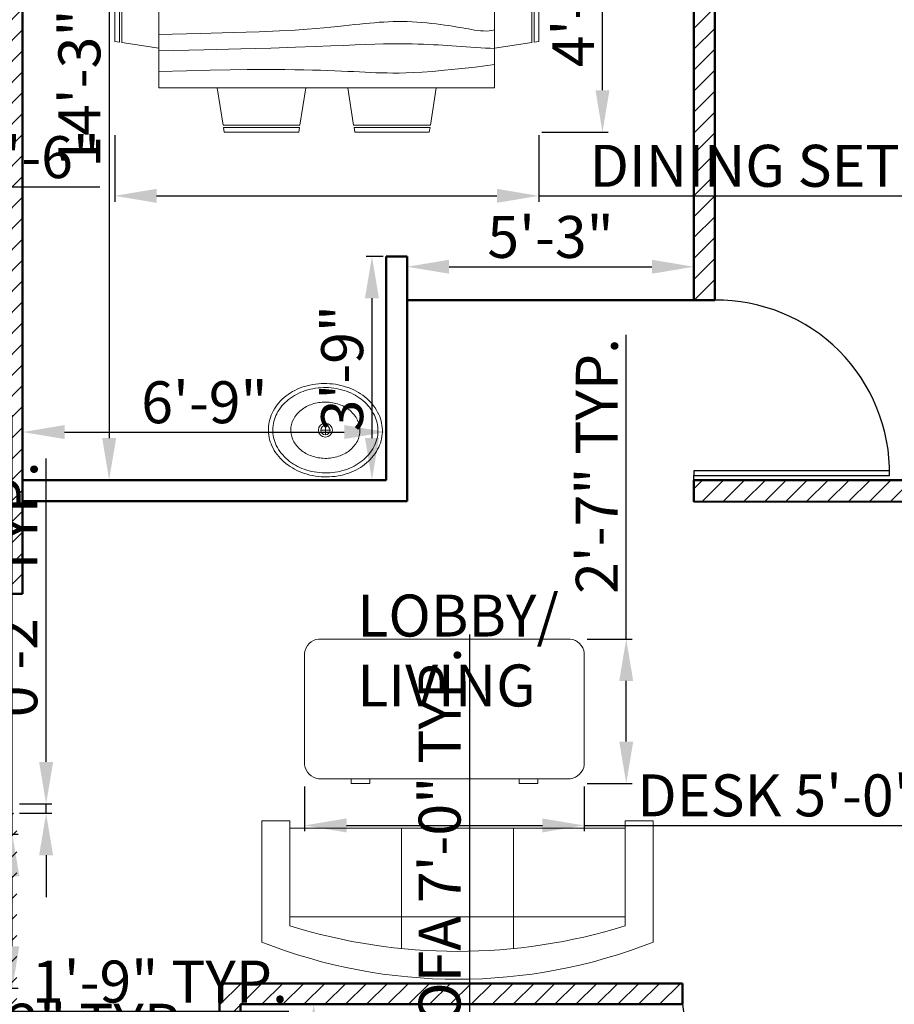
# Model space of a CAD drawing. Units: inches. Extents: x 5928 to 6612, y 5674 to 6320.
# Tile 3 of 5: x 6219 to 6407, y 5862 to 6074. Entities that reach past the tile are written whole.
import ezdxf

# ---------------------------------------------------------------- set-up
doc = ezdxf.new("R2010")
doc.units = ezdxf.units.IN
for name, color, linetype, lineweight in [('A-ANNO-DIMS', 2, 'Continuous', 18), ('A-AREA-IDEN', 7, 'Continuous', 25), ('A-DOOR', 3, 'Continuous', 25), ('A-FLOR-FIXT', 9, 'Continuous', 18), ('A-FURN', 8, 'Continuous', 18), ('A-WALL', 7, 'Continuous', 50), ('A-WALL-PATT', 252, 'Continuous', 13)]:
    doc.layers.add(name, color=color, linetype=linetype, lineweight=lineweight)
doc.styles.get("Standard").update_dxf_attribs({"font": 'arial.ttf'})
doc.dimstyles.new('ISO-25', dxfattribs={"dimtxt": 9, "dimasz": 9, "dimexe": 1.25, "dimexo": 0.625, "dimtad": 1, "dimdec": 1, "dimrnd": 9, "dimlunit": 3, "dimtxsty": 'Standard', "dimcen": 2.5, "dimadec": 0, "dimazin": 0, "dimtfac": 1, "dimtdec": 1, "dimtmove": 0, "dimatfit": 3, "dimfxl": 1, "dimarcsym": 0})

# ---------------------------------------------------------------- blocks, each defined once
blk = doc.blocks.new('Dining Set - 36 x 72 in.')
for p, q in [((-22, 27.5), (-22.1562, 26.50042)), ((-22, 27.5), (-6, 27.5)), ((-5.8437, 26.49966), (-6, 27.5)), ((6, 27.5), (5.8438, 26.50042)), ((6, 27.5), (22, 27.5)), ((22.1563, 26.49966), (22, 27.5)), ((-22.2343, 26.00059), (-23.4847, 17.99762)), ((-22.2304, 26), (-5.7608, 26)), ((-5.8416, 26.5), (-22.1534, 26.5)), ((-4.5152, 17.99762), (-5.7655, 25.99926)), ((5.7657, 26.00059), (4.5153, 17.99762)), ((5.7696, 26), (22.2392, 26)), ((22.1584, 26.5), (5.8466, 26.5)), ((23.4848, 17.99762), (22.2345, 25.99926)), ((36, 18), (-36, 18)), ((-36, 18), (-36, -18)), ((36, -18), (36, 18)), ((-44.0006, 8.23428), (-35.9976, 9.48474)), ((44.0006, 8.23428), (35.9976, 9.48474)), ((-45.5, 8), (-44.5004, 8.15617)), ((-45.5, 8), (-45.5, -8)), ((-44.5, -8.15843), (-44.5, 8.15338)), ((-44, 8.23041), (-44, -8.23915)), ((44, 8.23041), (44, -8.23915)), ((44.5, -8.15843), (44.5, 8.15338)), ((45.5, 8), (44.5005, 8.15617)), ((45.5, 8), (45.5, -8)), ((-44.4997, -8.15631), (-45.5, -8)), ((-35.9976, -9.48476), (-43.9993, -8.2345)), ((35.9976, -9.48476), (43.9993, -8.2345)), ((44.4997, -8.15631), (45.5, -8)), ((-36, -18), (36, -18)), ((-22.2343, -26.0006), (-23.4847, -17.99762)), ((-4.5152, -17.99762), (-5.7655, -25.99928)), ((5.7657, -26.0006), (4.5153, -17.99762)), ((23.4848, -17.99762), (22.2345, -25.99928)), ((-22.2304, -26), (-5.7608, -26)), ((-22, -27.5), (-22.1562, -26.50044)), ((-5.8416, -26.5), (-22.1534, -26.5)), ((-5.8437, -26.49967), (-6, -27.5)), ((5.7696, -26), (22.2392, -26)), ((6, -27.5), (5.8438, -26.50044)), ((22.1584, -26.5), (5.8466, -26.5)), ((22.1563, -26.49967), (22, -27.5)), ((-22, -27.5), (-6, -27.5)), ((6, -27.5), (22, -27.5))]:
    blk.add_line(p, q)
for points in [[(-36, 15), (-31.1772, 14.97754), (-26.8079, 14.91406), (-22.8538, 14.81543), (-19.276, 14.6875), (-16.0362, 14.53613), (-13.0957, 14.36718), (-10.4159, 14.18652), (-7.9583, 14), (-5.6904, 13.81315), (-3.6035, 13.63021), (-1.6954, 13.45508), (0.0365, 13.29166), (1.5945, 13.14388), (2.9811, 13.01562), (4.1988, 12.9108), (5.25, 12.83333), (6.1393, 12.78613), (6.8802, 12.76823), (7.4883, 12.77767), (7.9792, 12.8125), (8.3685, 12.87077), (8.6719, 12.95052), (8.9049, 13.0498), (9.0833, 13.16666), (9.2205, 13.29899), (9.3216, 13.44401), (9.3895, 13.59879), (9.4271, 13.76041), (9.4373, 13.92594), (9.4232, 14.09245), (9.3875, 14.257), (9.3333, 14.41666), (9.2638, 14.56917), (9.1836, 14.71484), (9.0975, 14.85465), (9.0104, 14.98958), (8.9272, 15.1206), (8.8529, 15.2487), (8.7922, 15.37483), (8.75, 15.5), (8.7305, 15.62467), (8.7344, 15.74739), (8.7617, 15.86621), (8.8125, 15.97916), (8.8867, 16.08431), (8.9844, 16.17968), (9.1055, 16.26334), (9.25, 16.33333), (9.4189, 16.38802), (9.6172, 16.42708), (9.8506, 16.45052), (10.125, 16.45833), (10.4463, 16.45052), (10.8203, 16.42708), (11.2529, 16.38802), (11.75, 16.33333), (12.3184, 16.26318), (12.9694, 16.17838), (13.7151, 16.07991), (14.5677, 15.96875), (15.5395, 15.84586), (16.6426, 15.71224), (17.8893, 15.56884), (19.2917, 15.41666), (20.859, 15.25667), (22.5879, 15.08984), (24.4721, 14.91715), (26.5052, 14.73958), (28.6809, 14.5581), (30.9929, 14.3737), (33.4347, 14.18733), (36, 14)], [(-36, 10), (-28.9766, 10.14274), (-23.1725, 10.20442), (-18.4241, 10.19775), (-14.5677, 10.13541), (-11.4399, 10.03011), (-8.877, 9.89453), (-6.7154, 9.74137), (-4.7917, 9.58333), (-2.9698, 9.43082), (-1.2246, 9.28515), (0.4415, 9.14534), (2.026, 9.01041), (3.5266, 8.87939), (4.9408, 8.7513), (6.266, 8.62516), (7.5, 8.5), (8.6411, 8.37549), (9.6914, 8.2539), (10.6538, 8.13818), (11.5312, 8.03125), (12.3267, 7.93603), (13.043, 7.85547), (13.6831, 7.79248), (14.25, 7.75), (14.7471, 7.7303), (15.1797, 7.73307), (15.5537, 7.75732), (15.875, 7.80208), (16.1494, 7.86637), (16.3828, 7.94922), (16.5811, 8.04964), (16.75, 8.16666), (16.8944, 8.29915), (17.0143, 8.44531), (17.1089, 8.60319), (17.1771, 8.77083), (17.218, 8.94629), (17.2305, 9.1276), (17.2137, 9.31282), (17.1667, 9.5), (17.0895, 9.6875), (16.987, 9.875), (16.8649, 10.0625), (16.7292, 10.25), (16.5856, 10.4375), (16.4401, 10.625), (16.2985, 10.8125), (16.1667, 11), (16.05, 11.18733), (15.9518, 11.3737), (15.8752, 11.5581), (15.8229, 11.73958), (15.798, 11.91715), (15.8034, 12.08984), (15.842, 12.25667), (15.9167, 12.41666), (16.0295, 12.56836), (16.1784, 12.70833), (16.3605, 12.83268), (16.5729, 12.9375), (16.8127, 13.01888), (17.0768, 13.07291), (17.3625, 13.0957), (17.6667, 13.08333), (17.9894, 13.03312), (18.3418, 12.94726), (18.7382, 12.82918), (19.1927, 12.68229), (19.7195, 12.51001), (20.3327, 12.31575), (21.0465, 12.10294), (21.875, 11.875), (22.8357, 11.63354), (23.959, 11.37304), (25.2786, 11.08618), (26.8282, 10.76562), (28.6414, 10.40405), (30.752, 9.99414), (33.1936, 9.52856), (36, 9)], [(-36, 5.5), (-30.7157, 5.3348), (-26.069, 5.20963), (-21.9946, 5.11767), (-18.4271, 5.05208), (-15.3009, 5.00602), (-12.5508, 4.97265), (-10.1112, 4.94515), (-7.9167, 4.91666), (-5.909, 4.88167), (-4.0586, 4.83984), (-2.3429, 4.79215), (-0.7396, 4.73958), (0.7739, 4.6831), (2.22, 4.6237), (3.6213, 4.56233), (5, 4.5), (6.373, 4.43782), (7.7344, 4.3776), (9.0723, 4.32129), (10.375, 4.27083), (11.6309, 4.22819), (12.8281, 4.19531), (13.9551, 4.17415), (15, 4.16666), (15.954, 4.17448), (16.819, 4.19791), (17.6001, 4.23698), (18.3021, 4.29166), (18.9299, 4.36198), (19.4883, 4.44791), (19.9823, 4.54948), (20.4167, 4.66666), (20.7969, 4.79899), (21.1302, 4.94401), (21.4245, 5.09879), (21.6875, 5.26041), (21.9271, 5.42594), (22.1511, 5.59245), (22.3672, 5.757), (22.5834, 5.91666), (22.8065, 6.06868), (23.0404, 6.21093), (23.2879, 6.34147), (23.5521, 6.45833), (23.8358, 6.55957), (24.142, 6.64323), (24.4735, 6.70735), (24.8334, 6.75), (25.2235, 6.76969), (25.642, 6.76692), (26.0858, 6.74267), (26.5521, 6.69791), (27.0379, 6.63362), (27.5404, 6.55078), (28.0565, 6.45036), (28.5834, 6.33333), (29.1242, 6.19987), (29.7071, 6.04687), (30.3661, 5.87044), (31.1354, 5.66666), (32.0493, 5.43164), (33.142, 5.16146), (34.4475, 4.85221), (36, 4.5)], [(-36, -1), (-30.7915, -0.6591), (-26.0195, -0.38216), (-21.6519, -0.16284), (-17.6563, 0.00521), (-14.0005, 0.12833), (-10.6523, 0.21289), (-7.5796, 0.26522), (-4.75, 0.29166), (-2.134, 0.29793), (0.2878, 0.28711), (2.5317, 0.26163), (4.6146, 0.22396), (6.5529, 0.17651), (8.3633, 0.12174), (10.0623, 0.06209), (11.6667, 0), (13.1899, -0.06201), (14.6341, -0.1211), (15.9982, -0.17432), (17.2813, -0.21875), (18.4823, -0.25147), (19.6003, -0.26953), (20.6343, -0.27002), (21.5834, -0.25), (22.4481, -0.20768), (23.2357, -0.14584), (23.9549, -0.06836), (24.6146, 0.02083), (25.2235, 0.11784), (25.7904, 0.21875), (26.3241, 0.31966), (26.8334, 0.41666), (27.3265, 0.50618), (27.8099, 0.58593), (28.2894, 0.65397), (28.7709, 0.70833), (29.2601, 0.74707), (29.763, 0.76823), (30.2855, 0.76985), (30.8334, 0.75), (31.4088, 0.70784), (31.9994, 0.64713), (32.589, 0.57275), (33.1615, 0.48958), (33.7008, 0.4025), (34.1908, 0.3164), (34.6153, 0.23616), (34.9584, 0.16666), (35.2099, 0.11165), (35.3848, 0.07031), (35.504, 0.04069), (35.5886, 0.02083), (35.6594, 0.00879), (35.7377, 0.0026), (35.8442, 0.00032), (36, 0)], [(-36, -6.5), (-27.1843, -6.31267), (-20.084, -6.1263), (-14.469, -5.9419), (-10.1094, -5.76042), (-6.7752, -5.58285), (-4.2363, -5.41016), (-2.2629, -5.24333), (-0.625, -5.08334), (0.8708, -4.93099), (2.2715, -4.78646), (3.5872, -4.64974), (4.8281, -4.52084), (6.0046, -4.39974), (7.127, -4.28646), (8.2053, -4.18099), (9.25, -4.08334), (10.2705, -3.99382), (11.2734, -3.91407), (12.2647, -3.84603), (13.25, -3.79167), (14.2354, -3.75293), (15.2266, -3.73177), (16.2295, -3.73015), (17.25, -3.75), (18.2912, -3.79248), (19.3451, -3.85547), (20.4009, -3.93604), (21.4479, -4.03125), (22.4754, -4.13819), (23.4727, -4.25391), (24.4289, -4.37549), (25.3334, -4.5), (26.1785, -4.62492), (26.9694, -4.74935), (27.7145, -4.87281), (28.4219, -4.99479), (29.1, -5.11483), (29.7572, -5.23242), (30.4016, -5.34709), (31.0417, -5.45834), (31.6837, -5.56437), (32.3262, -5.65821), (32.9658, -5.73153), (33.599, -5.77604), (34.2224, -5.78345), (34.8327, -5.74545), (35.4264, -5.65373), (36, -5.5)], [(-36, -10), (-26.4022, -9.81299), (-18.4675, -9.62891), (-11.9839, -9.45069), (-6.7396, -9.28125), (-2.5226, -9.12354), (0.8789, -8.98047), (3.6769, -8.85498), (6.0833, -8.75), (8.2767, -8.66765), (10.3021, -8.60677), (12.1712, -8.56543), (13.8958, -8.54167), (15.4876, -8.53353), (16.9583, -8.53907), (18.3197, -8.55632), (19.5834, -8.58334), (20.7616, -8.61841), (21.8685, -8.66081), (22.9188, -8.71004), (23.9271, -8.76563), (24.9081, -8.82707), (25.8763, -8.89388), (26.8465, -8.96558), (27.8334, -9.04167), (28.8474, -9.12118), (29.8828, -9.20117), (30.93, -9.27824), (31.9792, -9.34896), (33.0205, -9.40991), (34.0443, -9.45768), (35.0407, -9.48885), (36, -9.5)], [(-36, -14.5), (-30.0881, -14.33513), (-25.0332, -14.21224), (-20.7312, -14.12647), (-17.0781, -14.07292), (-13.97, -14.04671), (-11.3027, -14.04297), (-8.9724, -14.05681), (-6.875, -14.08334), (-4.9224, -14.11833), (-3.0905, -14.16016), (-1.3709, -14.20785), (0.2448, -14.26042), (1.7647, -14.3169), (3.1973, -14.3763), (4.5507, -14.43767), (5.8333, -14.5), (7.0554, -14.5621), (8.235, -14.62175), (9.3922, -14.67652), (10.5469, -14.72396), (11.7192, -14.76164), (12.929, -14.78711), (14.1965, -14.79794), (15.5417, -14.79167), (16.9933, -14.76424), (18.6152, -14.70508), (20.4804, -14.60197), (22.6615, -14.44271), (25.2312, -14.21509), (28.2624, -13.9069), (31.8277, -13.50594), (36, -13)]]:
    blk.add_lwpolyline(points)
blk = doc.blocks.new('Sofa - Roundback 7 ft.')
for p, q in [((-12.00002, -32.4421), (-12.00003, -6.5971)), ((11.99997, -32.4421), (11.99998, -6.5971)), ((-36.000027, -34), (-36.000027, -11.4696)), ((35.99998, -34), (35.99998, -11.4696)), ((-35.999844, -13.3819), (35.9998, -13.3819)), ((-36.000027, -32.4421), (35.99998, -32.4421))]:
    blk.add_line(p, q)
for points in [[(-36.000027, -34), (-42.000027, -34), (-42.000027, -8)], [(41.99998, -8), (41.99998, -34), (35.99998, -34)]]:
    blk.add_lwpolyline(points)
for centre, radius, start, end in [((0, -114.25), 114.25, 68.43141, 111.5686), ((-0.00001, -127.1968), 121.1968, 72.72033, 107.2797)]:
    blk.add_arc(centre, radius, start, end)
blk = doc.blocks.new('Desk - 30 x 60 in.')
for p, q in [((-26.999995, 0), (26.999995, 0)), ((-29.999995, -27), (-29.999995, -3)), ((29.999995, -3), (29.999995, -27)), ((26.999995, -30), (-26.999995, -30)), ((-20.000005, -30), (-20.000005, -31)), ((-20.000005, -31), (-16.000005, -31)), ((-16.000005, -31), (-16.000005, -30)), ((15.999995, -31), (15.999995, -30)), ((19.999995, -31), (15.999995, -31)), ((19.999995, -30), (19.999995, -31))]:
    blk.add_line(p, q)
for centre, start, end in [((-26.499995, -3.5), 98.1301, 171.8699), ((26.499995, -3.5), 8.130102, 81.8699), ((-26.499995, -26.5), 188.1301, 261.8699), ((26.499995, -26.5), 278.1301, 351.8699)]:
    blk.add_arc(centre, 3.535534, start, end)
blk = doc.blocks.new('Sink - Oval top')
for p, q in [((-1, 0), (1, 0)), ((0, 1), (0, -1))]:
    blk.add_line(p, q)
for points in [[(-12.23, 0.39, 0.117634), (-11.46, -3.36, 0.104469), (-8.88, -6.8, 0.090016), (-5.08, -9.07, 0.08192), (-0.32, -10.02, 0.08192), (4.49, -9.38, 0.090016), (8.42, -7.36, 0.104469), (11.22, -4.09, 0.117634), (12.23, -0.39, 0.117634), (11.46, 3.36, 0.104469), (8.88, 6.8, 0.090016), (5.08, 9.07, 0.08192), (0.32, 10.02, 0.08192), (-4.49, 9.38, 0.090016), (-8.42, 7.36, 0.104469), (-11.22, 4.09, 0.117634)], [(-11.29, 0.16, 0.118622), (-10.52, -3.25, 0.104678), (-8.07, -6.36, 0.089562), (-4.54, -8.37, 0.081185), (-0.13, -9.15, 0.081185), (4.3, -8.49, 0.089562), (7.89, -6.58, 0.104678), (10.42, -3.55, 0.118622), (11.29, -0.16, 0.118622), (10.52, 3.25, 0.104678), (8.07, 6.36, 0.089562), (4.54, 8.37, 0.081185), (0.13, 9.15, 0.081185), (-4.3, 8.49, 0.089562), (-7.89, 6.58, 0.104678), (-10.42, 3.55, 0.118622)], [(-7.42, 0.08, 0.118283), (-6.91, -2.17, 0.104607), (-5.29, -4.21, 0.089718), (-2.97, -5.53, 0.081436), (-0.07, -6.04, 0.081436), (2.84, -5.59, 0.089718), (5.2, -4.33, 0.104607), (6.86, -2.32, 0.118283), (7.42, -0.08, 0.118283), (6.91, 2.17, 0.104607), (5.29, 4.21, 0.089718), (2.97, 5.53, 0.081436), (0.07, 6.04, 0.081436), (-2.84, 5.59, 0.089718), (-5.2, 4.33, 0.104607), (-6.86, 2.32, 0.118283)]]:
    blk.add_lwpolyline(points, format="xyb", close=True)
for radius in [1.5, 1]:
    blk.add_circle((0, 0), radius)
blk = doc.blocks.new('*D21')
at = {"layer": 'A-ANNO-DIMS', "color": 0, "lineweight": -2, "transparency": 16777216}
for p, q in [((6266.88, 5862.26), (6283.21, 5862.26)), ((6281.96, 5853.26), (6281.96, 5729.26)), ((6266.88, 5720.26), (6283.21, 5720.26))]:
    blk.add_line(p, q, dxfattribs=at)
at = {"layer": 'A-ANNO-DIMS', "color": 0, "transparency": 16777216}
for points in [[(6280.46, 5853.26), (6283.46, 5853.26), (6281.96, 5862.26)], [(6280.46, 5729.26), (6283.46, 5729.26), (6281.96, 5720.26)]]:
    blk.add_solid(points, dxfattribs=at)
at = {"layer": 'Defpoints', "color": 0, "transparency": 16777216}
for p in [(6266.26, 5862.26), (6266.26, 5720.26), (6281.96, 5720.26)]:
    blk.add_point(p, dxfattribs=at)
at = {"layer": 'A-ANNO-DIMS', "color": 0, "transparency": 16777216, "insert": (6276.82, 5791.26), "char_height": 9, "attachment_point": 5, "rotation": 90}
blk.add_mtext("12'", dxfattribs=at)
blk = doc.blocks.new('*D23')
at = {"layer": 'A-ANNO-DIMS', "color": 0, "lineweight": -2, "transparency": 16777216}
for p, q in [((6220.15, 6142.76), (6239.34, 6142.76)), ((6238.09, 6133.76), (6238.09, 5983.76)), ((6220.15, 5974.76), (6239.34, 5974.76))]:
    blk.add_line(p, q, dxfattribs=at)
at = {"layer": 'A-ANNO-DIMS', "color": 0, "transparency": 16777216}
for points in [[(6236.59, 6133.76), (6239.59, 6133.76), (6238.09, 6142.76)], [(6236.59, 5983.76), (6239.59, 5983.76), (6238.09, 5974.76)]]:
    blk.add_solid(points, dxfattribs=at)
at = {"layer": 'Defpoints', "color": 0, "transparency": 16777216}
for p in [(6219.53, 6142.76), (6219.53, 5974.76), (6238.09, 5974.76)]:
    blk.add_point(p, dxfattribs=at)
at = {"layer": 'A-ANNO-DIMS', "color": 0, "transparency": 16777216, "insert": (6232.87, 6058.76), "char_height": 9, "attachment_point": 5, "rotation": 90}
blk.add_mtext('14\'-3"', dxfattribs=at)
blk = doc.blocks.new('*D24')
at = {"layer": 'A-ANNO-DIMS', "color": 0, "lineweight": -2, "transparency": 16777216}
for p, q in [((6219.53, 5975.39), (6219.53, 5986.31)), ((6297.53, 5975.39), (6297.53, 5986.31)), ((6228.53, 5985.06), (6288.53, 5985.06))]:
    blk.add_line(p, q, dxfattribs=at)
at = {"layer": 'A-ANNO-DIMS', "color": 0, "transparency": 16777216}
for points in [[(6228.53, 5986.56), (6228.53, 5983.56), (6219.53, 5985.06)], [(6288.53, 5986.56), (6288.53, 5983.56), (6297.53, 5985.06)]]:
    blk.add_solid(points, dxfattribs=at)
at = {"layer": 'Defpoints', "color": 0, "transparency": 16777216}
for p in [(6297.53, 5985.06), (6219.53, 5974.76), (6297.53, 5974.76)]:
    blk.add_point(p, dxfattribs=at)
at = {"layer": 'A-ANNO-DIMS', "color": 0, "transparency": 16777216, "insert": (6258.53, 5990.28), "char_height": 9, "attachment_point": 5}
blk.add_mtext('6\'-9"', dxfattribs=at)
blk = doc.blocks.new('*D25')
at = {"layer": 'A-ANNO-DIMS', "color": 0, "lineweight": -2, "transparency": 16777216}
for p, q in [((6296.9, 6022.76), (6293.21, 6022.76)), ((6294.46, 6013.76), (6294.46, 5983.76)), ((6296.9, 5974.76), (6293.21, 5974.76))]:
    blk.add_line(p, q, dxfattribs=at)
at = {"layer": 'A-ANNO-DIMS', "color": 0, "transparency": 16777216}
for points in [[(6292.96, 6013.76), (6295.96, 6013.76), (6294.46, 6022.76)], [(6292.96, 5983.76), (6295.96, 5983.76), (6294.46, 5974.76)]]:
    blk.add_solid(points, dxfattribs=at)
at = {"layer": 'Defpoints', "color": 0, "transparency": 16777216}
for p in [(6297.53, 6022.76), (6294.46, 5974.76), (6297.53, 5974.76)]:
    blk.add_point(p, dxfattribs=at)
at = {"layer": 'A-ANNO-DIMS', "color": 0, "transparency": 16777216, "insert": (6289.24, 5998.76), "char_height": 9, "attachment_point": 5, "rotation": 90}
blk.add_mtext('3\'-9"', dxfattribs=at)
blk = doc.blocks.new('*D26')
at = {"layer": 'A-ANNO-DIMS', "color": 0, "lineweight": -2, "transparency": 16777216}
for p, q in [((6302.03, 6022.14), (6302.03, 6019.28)), ((6363.53, 6022.14), (6363.53, 6019.28)), ((6311.03, 6020.53), (6354.53, 6020.53))]:
    blk.add_line(p, q, dxfattribs=at)
at = {"layer": 'A-ANNO-DIMS', "color": 0, "transparency": 16777216}
for points in [[(6311.03, 6022.03), (6311.03, 6019.03), (6302.03, 6020.53)], [(6354.53, 6022.03), (6354.53, 6019.03), (6363.53, 6020.53)]]:
    blk.add_solid(points, dxfattribs=at)
at = {"layer": 'Defpoints', "color": 0, "transparency": 16777216}
for p in [(6302.03, 6022.76), (6363.53, 6022.76), (6363.53, 6020.53)]:
    blk.add_point(p, dxfattribs=at)
at = {"layer": 'A-ANNO-DIMS', "color": 0, "transparency": 16777216, "insert": (6332.78, 6025.76), "char_height": 9, "attachment_point": 5}
blk.add_mtext('5\'-3"', dxfattribs=at)
blk = doc.blocks.new('DOOR-LEAF-42IN')
for p, q in [((0, 0), (0, 42)), ((0, 42), (1, 42)), ((1, 42), (1, 0)), ((-1, 0), (0, 0)), ((1, 0), (0, 0))]:
    blk.add_line(p, q)
blk = doc.blocks.new('*D45')
at = {"layer": 'A-ANNO-DIMS', "color": 0, "lineweight": -2, "transparency": 16777216}
for p, q in [((6224.56, 5914.26), (6224.56, 5979.37)), ((6218.88, 5905.26), (6225.81, 5905.26)), ((6224.56, 5903.26), (6224.56, 5905.26)), ((6218.88, 5903.26), (6225.81, 5903.26)), ((6224.56, 5894.26), (6224.56, 5885.26))]:
    blk.add_line(p, q, dxfattribs=at)
at = {"layer": 'A-ANNO-DIMS', "color": 0, "transparency": 16777216}
for points in [[(6223.06, 5914.26), (6226.06, 5914.26), (6224.56, 5905.26)], [(6223.06, 5894.26), (6226.06, 5894.26), (6224.56, 5903.26)]]:
    blk.add_solid(points, dxfattribs=at)
at = {"layer": 'Defpoints', "color": 0, "transparency": 16777216}
for p in [(6218.26, 5905.26), (6224.56, 5905.26), (6218.26, 5903.26)]:
    blk.add_point(p, dxfattribs=at)
at = {"layer": 'A-ANNO-DIMS', "color": 0, "transparency": 16777216, "insert": (6219.34, 5951.32), "char_height": 9, "attachment_point": 5, "rotation": 90}
blk.add_mtext('0\'-2" TYP.', dxfattribs=at)
blk = doc.blocks.new('*D48')
at = {"layer": 'A-ANNO-DIMS', "color": 0, "lineweight": -2, "transparency": 16777216}
for p, q in [((6217.31, 5898.76), (6217.31, 5988.68)), ((6212.98, 5898.76), (6218.56, 5898.76)), ((6217.31, 5874.72), (6217.31, 5889.76)), ((6212.98, 5865.72), (6218.56, 5865.72))]:
    blk.add_line(p, q, dxfattribs=at)
at = {"layer": 'A-ANNO-DIMS', "color": 0, "transparency": 16777216}
for points in [[(6215.81, 5889.76), (6218.81, 5889.76), (6217.31, 5898.76)], [(6215.81, 5874.72), (6218.81, 5874.72), (6217.31, 5865.72)]]:
    blk.add_solid(points, dxfattribs=at)
at = {"layer": 'Defpoints', "color": 0, "transparency": 16777216}
for p in [(6212.35, 5898.76), (6217.31, 5898.76), (6212.35, 5865.72)]:
    blk.add_point(p, dxfattribs=at)
at = {"layer": 'A-ANNO-DIMS', "color": 0, "transparency": 16777216, "insert": (6212.03, 5948.22), "char_height": 9, "attachment_point": 5, "rotation": 90}
blk.add_mtext('WC 2\'-9" TYP.', dxfattribs=at)
blk = doc.blocks.new('*D49')
at = {"layer": 'A-ANNO-DIMS', "color": 0, "lineweight": -2, "transparency": 16777216}
for p, q in [((6191.35, 5865.09), (6191.35, 5859.51)), ((6212.35, 5865.09), (6212.35, 5859.51)), ((6200.35, 5860.76), (6203.35, 5860.76)), ((6212.35, 5860.76), (6276.61, 5860.76))]:
    blk.add_line(p, q, dxfattribs=at)
at = {"layer": 'A-ANNO-DIMS', "color": 0, "transparency": 16777216}
for points in [[(6200.35, 5862.26), (6200.35, 5859.26), (6191.35, 5860.76)], [(6203.35, 5862.26), (6203.35, 5859.26), (6212.35, 5860.76)]]:
    blk.add_solid(points, dxfattribs=at)
at = {"layer": 'Defpoints', "color": 0, "transparency": 16777216}
for p in [(6191.35, 5865.72), (6212.35, 5865.72), (6212.35, 5860.76)]:
    blk.add_point(p, dxfattribs=at)
at = {"layer": 'A-ANNO-DIMS', "color": 0, "transparency": 16777216, "insert": (6248.98, 5865.98), "char_height": 9, "attachment_point": 5}
blk.add_mtext('1\'-9" TYP.', dxfattribs=at)
blk = doc.blocks.new('*D50')
at = {"layer": 'A-ANNO-DIMS', "color": 0, "lineweight": -2, "transparency": 16777216}
for p, q in [((6119.03, 6045.14), (6119.03, 6036.41)), ((6173.03, 6045.14), (6173.03, 6036.41)), ((6128.03, 6037.66), (6164.03, 6037.66)), ((6173.03, 6037.66), (6236.07, 6037.66))]:
    blk.add_line(p, q, dxfattribs=at)
at = {"layer": 'A-ANNO-DIMS', "color": 0, "transparency": 16777216}
for points in [[(6128.03, 6039.16), (6128.03, 6036.16), (6119.03, 6037.66)], [(6164.03, 6039.16), (6164.03, 6036.16), (6173.03, 6037.66)]]:
    blk.add_solid(points, dxfattribs=at)
at = {"layer": 'Defpoints', "color": 0, "transparency": 16777216}
for p in [(6119.03, 6045.76), (6173.03, 6045.76), (6173.03, 6037.66)]:
    blk.add_point(p, dxfattribs=at)
at = {"layer": 'A-ANNO-DIMS', "color": 0, "transparency": 16777216, "insert": (6209.05, 6042.88), "char_height": 9, "attachment_point": 5}
blk.add_mtext('TUB 4\'-6"', dxfattribs=at)
blk = doc.blocks.new('*D54')
at = {"layer": 'A-ANNO-DIMS', "color": 0, "lineweight": -2, "transparency": 16777216}
for p, q in [((6315.43, 5838.83), (6315.43, 5941.63)), ((6303.46, 5838.83), (6316.68, 5838.83)), ((6315.43, 5763.83), (6315.43, 5829.83)), ((6303.46, 5754.83), (6316.68, 5754.83))]:
    blk.add_line(p, q, dxfattribs=at)
at = {"layer": 'A-ANNO-DIMS', "color": 0, "transparency": 16777216}
for points in [[(6313.93, 5829.83), (6316.93, 5829.83), (6315.43, 5838.83)], [(6313.93, 5763.83), (6316.93, 5763.83), (6315.43, 5754.83)]]:
    blk.add_solid(points, dxfattribs=at)
at = {"layer": 'Defpoints', "color": 0, "transparency": 16777216}
for p in [(6302.83, 5838.83), (6315.43, 5838.83), (6302.83, 5754.83)]:
    blk.add_point(p, dxfattribs=at)
at = {"layer": 'A-ANNO-DIMS', "color": 0, "transparency": 16777216, "insert": (6310.15, 5894.73), "char_height": 9, "attachment_point": 5, "rotation": 90}
blk.add_mtext('SOFA 7\'-0" TYP.', dxfattribs=at)
blk = doc.blocks.new('*D55')
at = {"layer": 'A-ANNO-DIMS', "color": 0, "lineweight": -2, "transparency": 16777216}
for p, q in [((6266.17, 5839.46), (6266.17, 5852.68)), ((6302.83, 5839.46), (6302.83, 5852.68)), ((6266.17, 5851.43), (6180.09, 5851.43)), ((6293.83, 5851.43), (6275.17, 5851.43))]:
    blk.add_line(p, q, dxfattribs=at)
at = {"layer": 'A-ANNO-DIMS', "color": 0, "transparency": 16777216}
for points in [[(6275.17, 5852.93), (6275.17, 5849.93), (6266.17, 5851.43)], [(6293.83, 5852.93), (6293.83, 5849.93), (6302.83, 5851.43)]]:
    blk.add_solid(points, dxfattribs=at)
at = {"layer": 'Defpoints', "color": 0, "transparency": 16777216}
for p in [(6266.17, 5851.43), (6266.17, 5838.83), (6302.83, 5838.83)]:
    blk.add_point(p, dxfattribs=at)
at = {"layer": 'A-ANNO-DIMS', "color": 0, "transparency": 16777216, "insert": (6218.63, 5856.72), "char_height": 9, "attachment_point": 5, "rotation": 360}
blk.add_mtext('3\'-0 1/2" TYP.', dxfattribs=at)
blk = doc.blocks.new('*D56')
at = {"layer": 'A-ANNO-DIMS', "color": 0, "lineweight": -2, "transparency": 16777216}
for p, q in [((6280.02, 5909.02), (6280.02, 5899.4)), ((6340.02, 5909.02), (6340.02, 5899.4)), ((6289.02, 5900.65), (6331.02, 5900.65)), ((6340.02, 5900.65), (6442.41, 5900.65))]:
    blk.add_line(p, q, dxfattribs=at)
at = {"layer": 'A-ANNO-DIMS', "color": 0, "transparency": 16777216}
for points in [[(6289.02, 5902.15), (6289.02, 5899.15), (6280.02, 5900.65)], [(6331.02, 5902.15), (6331.02, 5899.15), (6340.02, 5900.65)]]:
    blk.add_solid(points, dxfattribs=at)
at = {"layer": 'Defpoints', "color": 0, "transparency": 16777216}
for p in [(6280.02, 5909.65), (6340.02, 5909.65), (6340.02, 5900.65)]:
    blk.add_point(p, dxfattribs=at)
at = {"layer": 'A-ANNO-DIMS', "color": 0, "transparency": 16777216, "insert": (6395.71, 5905.93), "char_height": 9, "attachment_point": 5}
blk.add_mtext('DESK 5\'-0" TYP.', dxfattribs=at)
blk = doc.blocks.new('*D57')
at = {"layer": 'A-ANNO-DIMS', "color": 0, "lineweight": -2, "transparency": 16777216}
for p, q in [((6349.02, 5940.65), (6349.02, 6005.91)), ((6340.64, 5940.65), (6350.27, 5940.65)), ((6349.02, 5918.65), (6349.02, 5931.65)), ((6340.64, 5909.65), (6350.27, 5909.65))]:
    blk.add_line(p, q, dxfattribs=at)
at = {"layer": 'A-ANNO-DIMS', "color": 0, "transparency": 16777216}
for points in [[(6347.52, 5931.65), (6350.52, 5931.65), (6349.02, 5940.65)], [(6347.52, 5918.65), (6350.52, 5918.65), (6349.02, 5909.65)]]:
    blk.add_solid(points, dxfattribs=at)
at = {"layer": 'Defpoints', "color": 0, "transparency": 16777216}
for p in [(6340.02, 5940.65), (6349.02, 5940.65), (6340.02, 5909.65)]:
    blk.add_point(p, dxfattribs=at)
at = {"layer": 'A-ANNO-DIMS', "color": 0, "transparency": 16777216, "insert": (6343.87, 5977.78), "char_height": 9, "attachment_point": 5, "rotation": 90}
blk.add_mtext('2\'-7" TYP.', dxfattribs=at)
blk = doc.blocks.new('*D64')
at = {"layer": 'A-ANNO-DIMS', "color": 0, "lineweight": -2, "transparency": 16777216}
for p, q in [((6239.27, 6048.77), (6239.27, 6034.49)), ((6330.27, 6048.77), (6330.27, 6034.49)), ((6248.27, 6035.74), (6321.27, 6035.74)), ((6330.27, 6035.74), (6439.44, 6035.74))]:
    blk.add_line(p, q, dxfattribs=at)
at = {"layer": 'A-ANNO-DIMS', "color": 0, "transparency": 16777216}
for points in [[(6248.27, 6037.24), (6248.27, 6034.24), (6239.27, 6035.74)], [(6321.27, 6037.24), (6321.27, 6034.24), (6330.27, 6035.74)]]:
    blk.add_solid(points, dxfattribs=at)
at = {"layer": 'Defpoints', "color": 0, "transparency": 16777216}
for p in [(6239.27, 6049.39), (6330.27, 6049.39), (6330.27, 6035.74)]:
    blk.add_point(p, dxfattribs=at)
at = {"layer": 'A-ANNO-DIMS', "color": 0, "transparency": 16777216, "insert": (6389.36, 6041.02), "char_height": 9, "attachment_point": 5}
blk.add_mtext('DINING SET 7\'-7"', dxfattribs=at)
blk = doc.blocks.new('*D65')
at = {"layer": 'A-ANNO-DIMS', "color": 0, "lineweight": -2, "transparency": 16777216}
for p, q in [((6330.9, 6104.39), (6345.17, 6104.39)), ((6343.92, 6058.39), (6343.92, 6095.39)), ((6330.9, 6049.39), (6345.17, 6049.39))]:
    blk.add_line(p, q, dxfattribs=at)
at = {"layer": 'A-ANNO-DIMS', "color": 0, "transparency": 16777216}
for points in [[(6342.42, 6095.39), (6345.42, 6095.39), (6343.92, 6104.39)], [(6342.42, 6058.39), (6345.42, 6058.39), (6343.92, 6049.39)]]:
    blk.add_solid(points, dxfattribs=at)
at = {"layer": 'Defpoints', "color": 0, "transparency": 16777216}
for p in [(6330.27, 6104.39), (6343.92, 6104.39), (6330.27, 6049.39)]:
    blk.add_point(p, dxfattribs=at)
at = {"layer": 'A-ANNO-DIMS', "color": 0, "transparency": 16777216, "insert": (6338.8, 6076.89), "char_height": 9, "attachment_point": 5, "rotation": 90}
blk.add_mtext('4\'-7"', dxfattribs=at)

msp = doc.modelspace()

# ---------------------------------------------------------------- hatches: boundary and pattern name
at = {"layer": 'A-WALL-PATT'}
h = msp.add_hatch(dxfattribs=at)
h.set_pattern_fill('ANSI31', color=256)
h.paths.add_polyline_path([(6071.03, 6165.76), (6215.03, 6165.76), (6215.03, 5969.77), (6215.03, 5950.32), (6219.53, 5950.32), (6219.53, 6142.76), (6239.11, 6142.76), (6239.11, 6151.76), (6224.03, 6151.76), (6224.03, 6174.76), (6062.03, 6174.76), (6062.03, 5969.76), (6062.03, 5894.26), (6108.76, 5894.26), (6108.76, 5711.26), (6423.76, 5711.26), (6423.76, 5750.35), (6414.76, 5750.35), (6414.76, 5720.26), (6266.26, 5720.26), (6266.26, 5862.26), (6361.1, 5862.26), (6361.1, 5866.76), (6261.76, 5866.76), (6261.76, 5720.26), (6117.76, 5720.26), (6117.76, 5792.26), (6218.26, 5792.26), (6218.26, 5796.76), (6117.76, 5796.76), (6117.76, 5898.76), (6213.76, 5898.76), (6213.76, 5828.21, -0.018207), (6216.01, 5828.09), (6218.26, 5828.09), (6218.26, 5903.26), (6117.76, 5903.26), (6071.03, 5903.26), (6071.03, 5969.77), (6071.03, 6041.26), (6117.76, 6041.26), (6172.44, 6041.26), (6172.44, 6045.76), (6117.76, 6045.76), (6071.03, 6045.76)])
h.paths.add_polyline_path([(6368.03, 6219.26), (6488.03, 6219.26), (6488.03, 6147.26), (6403.79, 6147.26), (6403.79, 6142.76), (6488.03, 6142.76), (6488.03, 5974.76), (6363.53, 5974.76), (6363.53, 5970.11), (6497.03, 5970.26), (6497.03, 6142.76), (6497.03, 6228.26), (6359.03, 6228.26), (6359.03, 6151.76), (6344.11, 6151.76), (6344.11, 6142.76), (6363.53, 6142.76), (6363.53, 6013.35), (6368.03, 6013.35), (6368.03, 6142.76)])
h.paths.add_polyline_path([(6344.11, 6196.21, 0.265753), (6295.16, 6228.26), (6288.06, 6228.26, 0.265753), (6239.11, 6196.21), (6239.11, 6142.76), (6243.61, 6142.76), (6243.61, 6196.76), (6243.45, 6196.76, -0.514089), (6339.79, 6196.74), (6339.61, 6196.76), (6339.61, 6142.76), (6344.11, 6142.76)])
h.paths.add_polyline_path([(6339.61, 6147.26), (6327.61, 6147.26), (6327.61, 6142.76), (6339.61, 6142.76)], flags=17)
h.paths.add_polyline_path([(6255.61, 6147.26), (6243.61, 6147.26), (6243.61, 6142.76), (6255.61, 6142.76)], flags=17)
h.paths.add_polyline_path([(6548.03, 5974.76), (6539.03, 5974.76), (6539.03, 5862.26), (6407.03, 5862.26), (6407.03, 5853.26), (6414.76, 5853.26), (6414.76, 5820.79), (6423.76, 5820.79), (6423.76, 5853.26), (6548.03, 5853.26)])

# ---------------------------------------------------------------- linework, layer by layer
at = {"layer": 'A-DOOR'}
for centre, radius, start, end in [((6368.44, 5976.26), 37.09, 359.2275, 90.6432), ((6405.53, 5866.89), 44.67, 185.9456, 270.6414)]:
    msp.add_arc(centre, radius, start, end, dxfattribs=at)
at = {"layer": 'A-WALL'}
for p, q in [((6219.53, 6142.76), (6219.53, 5950.32)), ((6363.53, 6013.35), (6363.53, 6142.76)), ((6368.03, 6013.35), (6368.03, 6142.76)), ((6302.03, 6022.76), (6297.53, 6022.76)), ((6297.53, 6022.76), (6297.53, 5974.76)), ((6302.03, 6022.76), (6302.03, 5970.26)), ((6368.03, 6013.35), (6302.03, 6013.35)), ((6297.53, 5974.76), (6219.53, 5974.76)), ((6488.03, 5974.76), (6363.53, 5974.76)), ((6363.53, 5974.76), (6363.53, 5970.11)), ((6302.03, 5970.26), (6219.53, 5970.26)), ((6497.03, 5970.26), (6363.53, 5970.11)), ((6215.03, 5950.32), (6219.53, 5950.32)), ((6261.76, 5866.76), (6261.76, 5720.26)), ((6361.1, 5866.76), (6261.76, 5866.76)), ((6361.1, 5866.76), (6361.1, 5862.26)), ((6361.1, 5862.26), (6266.26, 5862.26)), ((6266.26, 5862.26), (6266.26, 5720.26))]:
    msp.add_line(p, q, dxfattribs=at)

# ---------------------------------------------------------------- block references
at = {"layer": 'A-DOOR', "extrusion": (0, 0, -1), "zscale": -1, "rotation": 90.00000000000202}
msp.add_blockref('DOOR-LEAF-42IN', (-6363.53, 5975.76), dxfattribs=at)
at = {"layer": 'A-FLOR-FIXT'}
msp.add_blockref('Sink - Oval top', (6284.47, 5985.45), dxfattribs=at)
at = {"layer": 'A-FURN'}
for name, p in [('Dining Set - 36 x 72 in.', (6284.77, 6076.89)), ('Desk - 30 x 60 in.', (6310.02, 5940.65))]:
    msp.add_blockref(name, p, dxfattribs=at)
at = {"layer": 'A-FURN', "rotation": 179.9999744495946}
msp.add_blockref('Sofa - Roundback 7 ft.', (6312.82, 5867.63), dxfattribs=at)

# ---------------------------------------------------------------- texts
at = {"layer": 'A-AREA-IDEN', "insert": (6291.32, 5950.18), "char_height": 9, "attachment_point": 1}
msp.add_mtext_dynamic_manual_height_columns('LOBBY/\\PLIVING', width=64.9053, gutter_width=12.5, heights=[0], dxfattribs=at)

# ---------------------------------------------------------------- dimensions: what is measured, and where the dimension line sits
at = {"layer": 'A-ANNO-DIMS'}
for base, p1, p2, override, picture, middle in [((6238.09, 5974.76), (6219.53, 6142.76), (6219.53, 5974.76), {"dimclrd": 0, "dimclre": 0, "dimclrt": 0}, '*D23', (6232.87, 6058.76)), ((6343.92, 6104.39), (6330.27, 6049.39), (6330.27, 6104.39), {"dimdec": 1, "dimlfac": 1, "dimrnd": 0, "dimzin": 1, "dimdsep": 46, "dimlunit": 4, "dimfrac": 2}, '*D65', (6338.8, 6076.89)), ((6294.46, 5974.76), (6297.53, 6022.76), (6297.53, 5974.76), {"dimclrd": 0, "dimclre": 0, "dimclrt": 0}, '*D25', (6289.24, 5998.76)), ((6281.96, 5720.26), (6266.26, 5862.26), (6266.26, 5720.26), {"dimclrd": 0, "dimclre": 0, "dimclrt": 0}, '*D21', (6276.82, 5791.26))]:
    dim = msp.add_linear_dim(base=base, p1=p1, p2=p2, angle=90, dimstyle='ISO-25', override=override, dxfattribs=at)
    dim.commit()
    dim.dimension.update_dxf_attribs({"geometry": picture, "text_midpoint": middle})
for base, p1, p2, text, picture, middle in [((6330.27, 6035.74), (6239.27, 6049.39), (6330.27, 6049.39), 'DINING SET <>', '*D64', (6389.36, 6041.02)), ((6173.03, 6037.66), (6119.03, 6045.76), (6173.03, 6045.76), 'TUB <>', '*D50', (6209.05, 6042.88)), ((6340.02, 5900.65), (6280.02, 5909.65), (6340.02, 5909.65), 'DESK <> TYP.', '*D56', (6395.71, 5905.93)), ((6212.35, 5860.76), (6191.35, 5865.72), (6212.35, 5865.72), '<> TYP.', '*D49', (6248.98, 5865.98))]:
    dim = msp.add_linear_dim(base=base, p1=p1, p2=p2, text=text, dimstyle='ISO-25', override={"dimdec": 1, "dimlfac": 1, "dimrnd": 0, "dimzin": 1, "dimdsep": 46, "dimlunit": 4, "dimfrac": 2}, dxfattribs=at)
    dim.commit()
    dim.dimension.update_dxf_attribs({"geometry": picture, "text_midpoint": middle})
for base, p1, p2, picture, middle in [((6363.53, 6020.53), (6302.03, 6022.76), (6363.53, 6022.76), '*D26', (6332.78, 6025.76)), ((6297.53, 5985.06), (6219.53, 5974.76), (6297.53, 5974.76), '*D24', (6258.53, 5990.28))]:
    dim = msp.add_linear_dim(base=base, p1=p1, p2=p2, dimstyle='ISO-25', override={"dimclrd": 0, "dimclre": 0, "dimclrt": 0}, dxfattribs=at)
    dim.commit()
    dim.dimension.update_dxf_attribs({"geometry": picture, "text_midpoint": middle})
for base, p1, p2, angle, text, picture, middle in [((6349.02, 5940.65), (6340.02, 5909.65), (6340.02, 5940.65), 90, '<> TYP.', '*D57', (6343.87, 5977.78)), ((6217.31, 5898.76), (6212.35, 5865.72), (6212.35, 5898.76), 90, 'WC <> TYP.', '*D48', (6212.03, 5948.22)), ((6224.56, 5905.26), (6218.26, 5903.26), (6218.26, 5905.26), 90, '<> TYP.', '*D45', (6219.34, 5951.32)), ((6315.43, 5838.83), (6302.83, 5754.83), (6302.83, 5838.83), 90, 'SOFA <> TYP.', '*D54', (6310.15, 5894.73)), ((6266.17, 5851.43), (6302.83, 5838.83), (6266.17, 5838.83), 180, '<> TYP.', '*D55', (6218.63, 5856.72))]:
    dim = msp.add_linear_dim(base=base, p1=p1, p2=p2, angle=angle, text=text, dimstyle='ISO-25', override={"dimdec": 1, "dimlfac": 1, "dimrnd": 0, "dimzin": 1, "dimdsep": 46, "dimlunit": 4, "dimfrac": 2}, dxfattribs=at)
    dim.commit()
    dim.dimension.update_dxf_attribs({"geometry": picture, "text_midpoint": middle})

doc.saveas('drawing.dxf')
